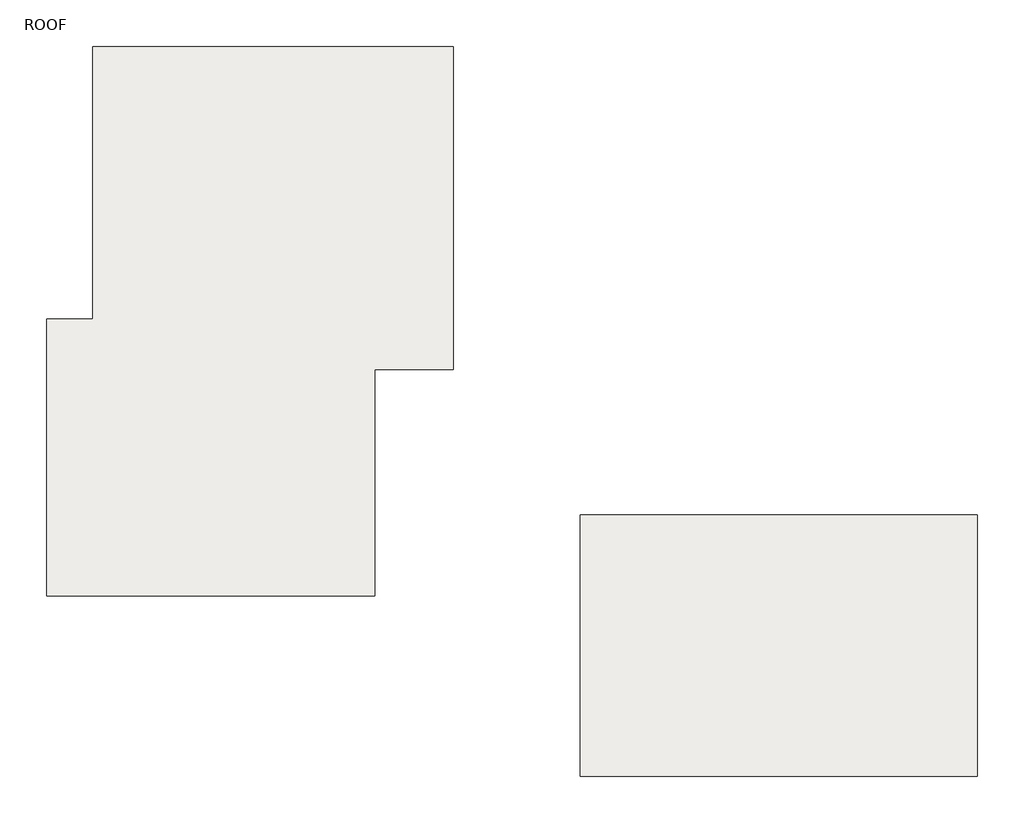
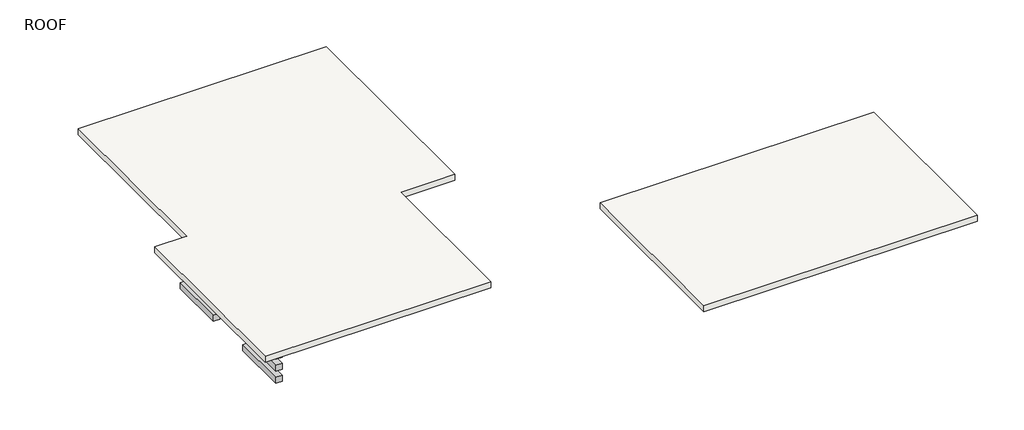
# One storey: 4 proxies, 2 slabs.
"""IFC4 building model written with IfcOpenShell, lengths in millimetres."""

from ifc_helpers import new_model, si_unit, frame, origin, place, context, project, spatial, polyline, outline, extrude, element, save

model = new_model("IFC4")

# Units and contexts
model_context = context("Model", 3, world=origin())
ifc_project = project(units=[si_unit("LENGTHUNIT", "METRE", prefix="MILLI")], contexts=[model_context])

# Site, building, storey
site = spatial("IfcSite", under=ifc_project)
building = spatial("IfcBuilding", under=site)
storey = spatial("IfcBuildingStorey", under=building, Name="ROOF", Elevation=16002.0)

# Proxies
placement = place(None, origin())
element("IfcBuildingElementProxy", 1, Name="Reveal", ObjectType="Reveal", at=placement, inside=storey, context=model_context, shape_type="SweptSolid", body=[
    extrude(outline(polyline([(-7008.3415084, 1592.333346), (-6855.9415084, 1592.333346), (-6855.9415084, 220.733346), (-7008.3415084, 220.733346), (-7008.3415084, 1592.333346)])), frame((0.0, 0.0, 14732.0), z_axis=(0.0, 0.0, 1.0), x_axis=(1.0, 0.0, 0.0)), (0.0, 0.0, 1.0), 152.4),
    extrude(outline(polyline([(-7008.3415084, 4183.133346), (-6855.9415084, 4183.133346), (-6855.9415084, 2811.533346), (-7008.3415084, 2811.533346), (-7008.3415084, 4183.133346)])), frame((0.0, 0.0, 14732.0), z_axis=(0.0, 0.0, 1.0), x_axis=(1.0, 0.0, 0.0)), (0.0, 0.0, 1.0), 152.4),
])
element("IfcBuildingElementProxy", 2, Name="Reveal", ObjectType="Reveal", at=placement, inside=storey, context=model_context, shape_type="SweptSolid", body=[
    extrude(outline(polyline([(-7008.3415084, 4183.133346), (-6855.9415084, 4183.133346), (-6855.9415084, 220.733346), (-7008.3415084, 220.733346), (-7008.3415084, 4183.133346)])), frame((0.0, 0.0, 15036.8), z_axis=(0.0, 0.0, 1.0), x_axis=(1.0, 0.0, 0.0)), (0.0, 0.0, 1.0), 152.4),
])
element("IfcBuildingElementProxy", 3, Name="Reveal", ObjectType="Reveal", at=placement, inside=storey, context=model_context, shape_type="SweptSolid", body=[
    extrude(outline(polyline([(-7008.3415084, 4183.133346), (-6855.9415084, 4183.133346), (-6855.9415084, 220.733346), (-7008.3415084, 220.733346), (-7008.3415084, 4183.133346)])), frame((0.0, 0.0, 15341.6), z_axis=(0.0, 0.0, 1.0), x_axis=(1.0, 0.0, 0.0)), (0.0, 0.0, 1.0), 152.4),
])
element("IfcBuildingElementProxy", 4, Name="Reveal", ObjectType="Reveal", at=placement, inside=storey, context=model_context, shape_type="SweptSolid", body=[
    extrude(outline(polyline([(-7008.3415084, 4183.133346), (-6855.9415084, 4183.133346), (-6855.9415084, 220.733346), (-7008.3415084, 220.733346), (-7008.3415084, 4183.133346)])), frame((0.0, 0.0, 15621.0), z_axis=(0.0, 0.0, 1.0), x_axis=(1.0, 0.0, 0.0)), (0.0, 0.0, 1.0), 152.4),
])

# Slabs
element("IfcSlab", 5, ObjectType="6\"", at=placement, inside=storey, context=model_context, shape_type="SweptSolid", body=[
    extrude(outline(polyline([(7735.5750459, 947.173346), (7735.5750459, -3363.206654), (1182.3750459, -3363.206654), (1182.3750459, 947.173346), (7735.5750459, 947.173346)])), frame((0.0, 0.0, 15849.6), z_axis=(0.0, 0.0, 1.0), x_axis=(1.0, 0.0, 0.0)), (0.0, 0.0, 1.0), 152.4),
])
element("IfcSlab", 6, ObjectType="6\"", at=placement, inside=storey, context=model_context, shape_type="SweptSolid", body=[
    extrude(outline(polyline([(-6855.9415084, 8678.933346), (-912.3415084, 8678.933346), (-912.3415084, 3344.933346), (-2207.7415084, 3344.933346), (-2207.7415084, -388.866654), (-7617.9415084, -388.866654), (-7617.9415084, 4183.133346), (-6855.9415084, 4183.133346), (-6855.9415084, 8678.933346)])), frame((0.0, 0.0, 15849.6), z_axis=(0.0, 0.0, 1.0), x_axis=(1.0, 0.0, 0.0)), (0.0, 0.0, 1.0), 152.4),
])

save(model, "model.ifc")

# Revit data of these elements
# Type "6\""
#   Assembly Code = "B1010"
#   Function = 0
#   Layers, outside or top first: 0' - 6" no material (function 1)
# Element 5 (IfcSlab, "6\"")
#   Height Offset From Level = 0' - 0"
#   Phase Created = New Construction
#   Materials on its faces: "Default Floor", "WALL 4"
# Element 6 (IfcSlab, "6\"")
#   built-in parameter 1001955 = 1.5708 (stored number, unit not read)
#   Height Offset From Level = 0' - 0"
#   Phase Created = New Construction
#   Materials on its faces: "Default Floor", "WALL 4"
# Materials
#   "Default Floor": colour RGB 128 128 128, transparency 0, Cost = 0
#   "WALL 4": class "Generic", colour RGB 32 32 32, transparency 0, Cost = 0
